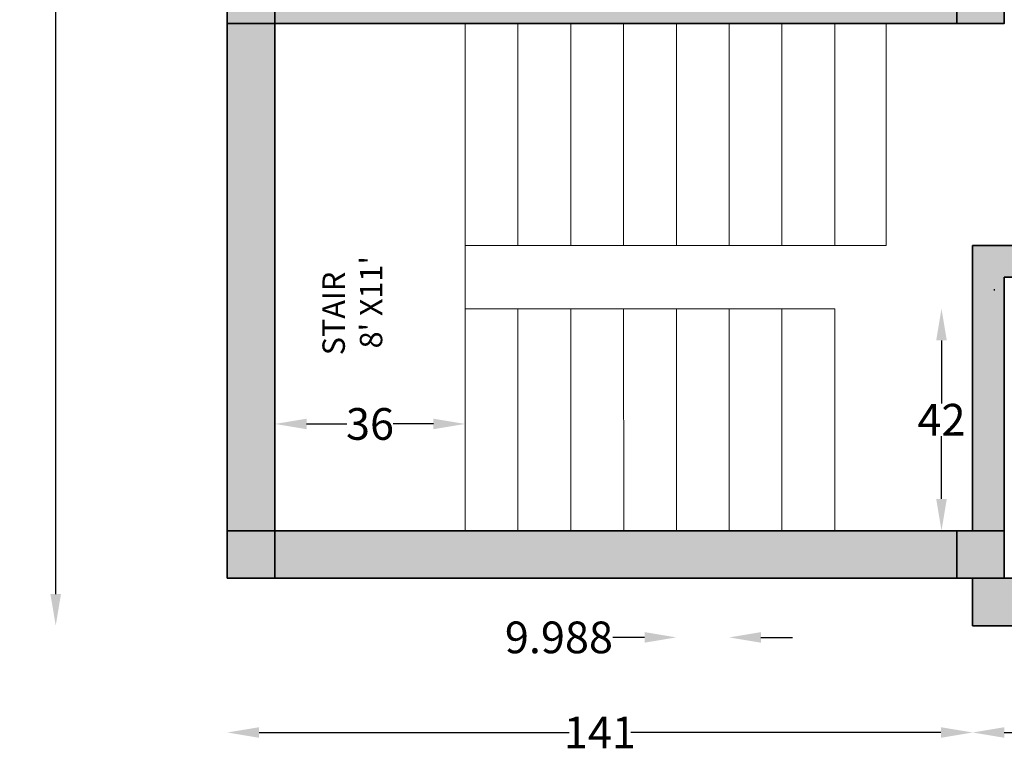
# Model space of a CAD drawing. Units: inches. Extents: x 1994 to 3075, y 3517 to 3950.
# Tile 48 of 58: x 2630 to 2816, y 3517 to 3656. Entities that reach past the tile are written whole.
import ezdxf

# ---------------------------------------------------------------- set-up
doc = ezdxf.new("R2010")
doc.units = ezdxf.units.IN
for name, color, linetype, lineweight in [('A-ANNO-DIMS', 2, 'Continuous', 18), ('A-AREA-IDEN', 7, 'Continuous', 18), ('A-COLS', 7, 'Continuous', 35), ('A-COLS-PATT', 6, 'Continuous', 13), ('A-FLOR-STRS', 7, 'Continuous', 18), ('A-WALL', 7, 'Continuous', 35), ('A-WALL-PATT', 252, 'Continuous', 13)]:
    doc.layers.add(name, color=color, linetype=linetype, lineweight=lineweight)
doc.styles.get("Standard").update_dxf_attribs({"font": 'arial.ttf'})
doc.dimstyles.get("Standard").update_dxf_attribs({"dimtxt": 6, "dimasz": 6, "dimexe": 0.18, "dimexo": 0.0625, "dimgap": 0.09, "dimtad": 0, "dimtih": 1, "dimtoh": 1, "dimdec": 4, "dimzin": 0, "dimdsep": 46, "dimlunit": 4, "dimtxsty": 'Standard', "dimcen": 0.09, "dimse1": 1, "dimse2": 1, "dimadec": 0, "dimazin": 0, "dimtfac": 1, "dimtdec": 4, "dimtofl": 0, "dimtmove": 0, "dimatfit": 3, "dimfxl": 1, "dimtolj": 1, "dimtzin": 0, "dimarcsym": 0})

# ---------------------------------------------------------------- blocks, each defined once
blk = doc.blocks.new('*D32')
at = {"layer": 'A-ANNO-DIMS', "color": 0, "lineweight": -2, "transparency": 16777216}
for p, q in [((2636.61, 3908.13), (2636.61, 3730.78)), ((2636.61, 3547.13), (2636.61, 3724.47))]:
    blk.add_line(p, q, dxfattribs=at)
at = {"layer": 'A-ANNO-DIMS', "color": 0, "transparency": 16777216}
for points in [[(2635.61, 3908.13), (2637.61, 3908.13), (2636.61, 3914.13)], [(2635.61, 3547.13), (2637.61, 3547.13), (2636.61, 3541.13)]]:
    blk.add_solid(points, dxfattribs=at)
at = {"layer": 'Defpoints', "color": 0, "transparency": 16777216}
for p in [(2636.61, 3914.13), (2669.07, 3914.13), (2810.07, 3541.13)]:
    blk.add_point(p, dxfattribs=at)
at = {"layer": 'A-ANNO-DIMS', "color": 0, "transparency": 16777216, "insert": (2636.61, 3727.63), "char_height": 6, "attachment_point": 5}
blk.add_mtext('\\A1;373', dxfattribs=at)
blk = doc.blocks.new('*D33')
at = {"layer": 'A-ANNO-DIMS', "color": 0, "lineweight": -2, "transparency": 16777216}
for p, q in [((2675.07, 3520.93), (2733.72, 3520.93)), ((2804.07, 3520.93), (2745.43, 3520.93))]:
    blk.add_line(p, q, dxfattribs=at)
at = {"layer": 'A-ANNO-DIMS', "color": 0, "transparency": 16777216}
for points in [[(2675.07, 3521.93), (2675.07, 3519.93), (2669.07, 3520.93)], [(2804.07, 3521.93), (2804.07, 3519.93), (2810.07, 3520.93)]]:
    blk.add_solid(points, dxfattribs=at)
at = {"layer": 'Defpoints', "color": 0, "transparency": 16777216}
for p in [(2669.07, 3550.13), (2810.07, 3541.13), (2810.07, 3520.93)]:
    blk.add_point(p, dxfattribs=at)
at = {"layer": 'A-ANNO-DIMS', "color": 0, "transparency": 16777216, "insert": (2739.57, 3520.93), "char_height": 6, "attachment_point": 5}
blk.add_mtext('\\A1;141', dxfattribs=at)
blk = doc.blocks.new('*D34')
at = {"layer": 'A-ANNO-DIMS', "color": 0, "lineweight": -2, "transparency": 16777216}
for p, q in [((2816.07, 3520.93), (2865.14, 3520.93)), ((2927.07, 3520.93), (2878.01, 3520.93))]:
    blk.add_line(p, q, dxfattribs=at)
at = {"layer": 'A-ANNO-DIMS', "color": 0, "transparency": 16777216}
for points in [[(2816.07, 3521.93), (2816.07, 3519.93), (2810.07, 3520.93)], [(2927.07, 3521.93), (2927.07, 3519.93), (2933.07, 3520.93)]]:
    blk.add_solid(points, dxfattribs=at)
at = {"layer": 'Defpoints', "color": 0, "transparency": 16777216}
for p in [(2810.07, 3541.13), (2933.07, 3541.13), (2933.07, 3520.93)]:
    blk.add_point(p, dxfattribs=at)
at = {"layer": 'A-ANNO-DIMS', "color": 0, "transparency": 16777216, "insert": (2871.57, 3520.93), "char_height": 6, "attachment_point": 5}
blk.add_mtext('\\A1;123', dxfattribs=at)
blk = doc.blocks.new('*D52')
at = {"layer": 'A-ANNO-DIMS', "color": 0, "lineweight": -2, "transparency": 16777216}
for p, q in [((2684.07, 3579.33), (2691.69, 3579.33)), ((2708.07, 3579.33), (2700.46, 3579.33))]:
    blk.add_line(p, q, dxfattribs=at)
at = {"layer": 'A-ANNO-DIMS', "color": 0, "transparency": 16777216}
for points in [[(2684.07, 3580.33), (2684.07, 3578.33), (2678.07, 3579.33)], [(2708.07, 3580.33), (2708.07, 3578.33), (2714.07, 3579.33)]]:
    blk.add_solid(points, dxfattribs=at)
at = {"layer": 'Defpoints', "color": 0, "transparency": 16777216}
for p in [(2714.07, 3579.33), (2678.07, 3559.13), (2714.07, 3559.13)]:
    blk.add_point(p, dxfattribs=at)
at = {"layer": 'A-ANNO-DIMS', "color": 0, "transparency": 16777216, "insert": (2696.07, 3579.33), "char_height": 6, "attachment_point": 5}
blk.add_mtext('\\A1;36', dxfattribs=at)
blk = doc.blocks.new('*D53')
at = {"layer": 'A-ANNO-DIMS', "color": 0, "lineweight": -2, "transparency": 16777216}
for p, q in [((2804.19, 3595.13), (2804.19, 3583.23)), ((2804.19, 3565.13), (2804.19, 3577.02))]:
    blk.add_line(p, q, dxfattribs=at)
at = {"layer": 'A-ANNO-DIMS', "color": 0, "transparency": 16777216}
for points in [[(2803.19, 3595.13), (2805.19, 3595.13), (2804.19, 3601.13)], [(2803.19, 3565.13), (2805.19, 3565.13), (2804.19, 3559.13)]]:
    blk.add_solid(points, dxfattribs=at)
at = {"layer": 'Defpoints', "color": 0, "transparency": 16777216}
for p in [(2783.99, 3601.13), (2783.99, 3559.13), (2804.19, 3559.13)]:
    blk.add_point(p, dxfattribs=at)
at = {"layer": 'A-ANNO-DIMS', "color": 0, "transparency": 16777216, "insert": (2804.19, 3580.13), "char_height": 6, "attachment_point": 5}
blk.add_mtext('\\A1;42', dxfattribs=at)
blk = doc.blocks.new('*D54')
at = {"layer": 'A-ANNO-DIMS', "color": 0, "lineweight": -2, "transparency": 16777216}
for p, q in [((2748.03, 3538.93), (2742.03, 3538.93)), ((2770.01, 3538.93), (2776.01, 3538.93))]:
    blk.add_line(p, q, dxfattribs=at)
at = {"layer": 'A-ANNO-DIMS', "color": 0, "transparency": 16777216}
for points in [[(2748.03, 3539.93), (2748.03, 3537.93), (2754.03, 3538.93)], [(2770.01, 3539.93), (2770.01, 3537.93), (2764.01, 3538.93)]]:
    blk.add_solid(points, dxfattribs=at)
at = {"layer": 'Defpoints', "color": 0, "transparency": 16777216}
for p in [(2754.03, 3559.13), (2764.01, 3559.13), (2754.03, 3538.93)]:
    blk.add_point(p, dxfattribs=at)
at = {"layer": 'A-ANNO-DIMS', "color": 0, "transparency": 16777216, "insert": (2731.81, 3538.93), "char_height": 6, "attachment_point": 5}
blk.add_mtext('\\A1;9.988', dxfattribs=at)
blk = doc.blocks.new('*D56')
at = {"layer": 'A-ANNO-DIMS', "color": 0, "lineweight": -2, "transparency": 16777216}
for p, q in [((2814.1, 3604.74), (2814.28, 3604.74)), ((2814.19, 3604.65), (2814.19, 3604.83)), ((2845.41, 3585.23), (2838.79, 3589.37)), ((2851.41, 3585.23), (2845.41, 3585.23))]:
    blk.add_line(p, q, dxfattribs=at)
at = {"layer": 'A-ANNO-DIMS', "color": 0, "transparency": 16777216}
blk.add_solid([(2839.32, 3590.22), (2838.26, 3588.52), (2833.7, 3592.55)], dxfattribs=at)
at = {"layer": 'Defpoints', "color": 0, "transparency": 16777216}
for p in [(2814.19, 3604.74), (2833.7, 3592.55)]:
    blk.add_point(p, dxfattribs=at)
at = {"layer": 'A-ANNO-DIMS', "color": 0, "transparency": 16777216, "insert": (2870.41, 3585.23), "char_height": 6, "attachment_point": 5}
blk.add_mtext('\\A1;2X R23.01', dxfattribs=at)

msp = doc.modelspace()

# ---------------------------------------------------------------- hatches: boundary and pattern name
at = {"layer": 'A-COLS-PATT'}
h = msp.add_hatch(color=256, dxfattribs=at)
h.dxf.hatch_style = 1
h.paths.add_polyline_path([(2678.072, 3914.1269), (2669.072, 3914.1269), (2669.072, 3905.1269), (2678.072, 3905.1269)])
h.paths.add_polyline_path([(2816.072, 3914.1269), (2807.072, 3914.1269), (2807.072, 3905.1269), (2816.072, 3905.1269)])
h.paths.add_polyline_path([(2894.9096, 3914.1269), (2885.9096, 3914.1269), (2885.9096, 3905.1269), (2894.9096, 3905.1269)])
h.paths.add_polyline_path([(3033.072, 3914.1269), (3024.072, 3914.1269), (3024.072, 3905.1269), (3033.072, 3905.1269)])
h.paths.add_polyline_path([(3033.072, 3764.1269), (3024.072, 3764.1269), (3024.072, 3755.1269), (3033.072, 3755.1269)])
h.paths.add_polyline_path([(2895.072, 3764.1269), (2886.072, 3764.1269), (2886.072, 3755.1269), (2895.072, 3755.1269)])
h.paths.add_polyline_path([(2816.072, 3764.1269), (2807.072, 3764.1269), (2807.072, 3755.1269), (2816.072, 3755.1269)])
h.paths.add_polyline_path([(2678.072, 3764.1269), (2669.072, 3764.1269), (2669.072, 3755.1269), (2678.072, 3755.1269)])
h.paths.add_polyline_path([(2678.072, 3664.1269), (2669.072, 3664.1269), (2669.072, 3655.1269), (2678.072, 3655.1269)])
h.paths.add_polyline_path([(2816.072, 3664.1269), (2807.072, 3664.1269), (2807.072, 3655.1269), (2816.072, 3655.1269)])
h.paths.add_polyline_path([(3033.072, 3616.1269), (3024.072, 3616.1269), (3024.072, 3607.1269), (3033.072, 3607.1269)])
h.paths.add_polyline_path([(2894.9096, 3616.1269), (2885.9096, 3616.1269), (2885.9096, 3607.1269), (2894.9096, 3607.1269)])
h.paths.add_polyline_path([(2816.072, 3559.1269), (2807.072, 3559.1269), (2807.072, 3550.1269), (2816.072, 3550.1269)])
h.paths.add_polyline_path([(2678.072, 3559.1269), (2669.072, 3559.1269), (2669.072, 3550.1269), (2678.072, 3550.1269)])
at = {"layer": 'A-WALL-PATT'}
h = msp.add_hatch(color=256, dxfattribs=at)
h.dxf.hatch_style = 1
h.paths.add_polyline_path([(2678.072, 3755.1269), (2669.072, 3755.1269), (2669.072, 3718.5523), (2678.072, 3718.5523)])
h.paths.add_polyline_path([(2807.072, 3761.1269), (2678.072, 3761.1269), (2678.072, 3755.1269), (2807.072, 3755.1269)])
h.paths.add_polyline_path([(2678.072, 3812.7371), (2669.072, 3812.7371), (2669.072, 3809.7371), (2669.072, 3764.1269), (2678.072, 3764.1269)])
h.paths.add_polyline_path([(2678.072, 3905.1269), (2669.072, 3905.1269), (2669.072, 3868.7491), (2678.072, 3868.7491)])
h.paths.add_polyline_path([(2723.826, 3914.1269), (2720.826, 3914.1269), (2678.072, 3914.1269), (2678.072, 3905.1269), (2723.826, 3905.1269)])
h.paths.add_polyline_path([(2807.072, 3914.1269), (2779.838, 3914.1269), (2779.838, 3905.1269), (2807.072, 3905.1269)])
h.paths.add_polyline_path([(2837.6979, 3914.1269), (2834.6979, 3914.1269), (2820.9062, 3914.1269), (2816.072, 3914.1269), (2816.072, 3905.1269), (2837.6979, 3905.1269)])
h.paths.add_polyline_path([(2885.9096, 3914.1269), (2869.71, 3914.1269), (2869.71, 3905.1269), (2876.9183, 3905.1269), (2885.9096, 3905.1269)])
h.paths.add_polyline_path([(2933.6904, 3914.1269), (2930.6904, 3914.1269), (2894.9096, 3914.1269), (2894.9096, 3905.1269), (2933.6904, 3905.1269)])
h.paths.add_polyline_path([(3024.072, 3914.1269), (2989.7025, 3914.1269), (2989.7025, 3905.1269), (3024.072, 3905.1269)])
h.paths.add_polyline_path([(3033.072, 3905.1269), (3024.072, 3905.1269), (3024.072, 3861.4192), (3033.072, 3861.4192)])
h.paths.add_polyline_path([(3033.072, 3805.4072), (3024.072, 3805.4072), (3024.072, 3764.1269), (3033.072, 3764.1269)])
h.paths.add_polyline_path([(3033.072, 3755.1269), (3024.072, 3755.1269), (3024.072, 3732.1247), (3033.072, 3732.1247), (3033.072, 3735.1247)])
h.paths.add_polyline_path([(3024.072, 3761.1269), (2895.072, 3761.1269), (2895.072, 3755.1269), (3024.072, 3755.1269)])
h.paths.add_polyline_path([(3033.072, 3676.1126), (3024.072, 3676.1126), (3024.072, 3616.1269), (3033.072, 3616.1269)])
h.paths.add_polyline_path([(3024.072, 3613.1269), (2959.4908, 3613.1269), (2959.4908, 3607.1269), (3024.072, 3607.1269)])
h.paths.add_polyline_path([(2914.1254, 3613.1269), (2894.9096, 3613.1269), (2894.9096, 3607.1269), (2914.1254, 3607.1269)])
h.paths.add_polyline_path([(2885.9096, 3613.1269), (2852.072, 3613.1269), (2852.072, 3607.1269), (2885.9096, 3607.1269)])
h.paths.add_polyline_path([(2822.072, 3613.1269), (2810.072, 3613.1269), (2810.072, 3559.1269), (2816.072, 3559.1269), (2816.072, 3607.1269), (2822.072, 3607.1269)])
h.paths.add_polyline_path([(2933.072, 3607.1269), (2924.072, 3607.1269), (2924.072, 3550.1269), (2892.072, 3550.1269), (2816.072, 3550.1269), (2810.072, 3550.1269), (2810.072, 3541.1269), (2892.072, 3541.1269), (2933.072, 3541.1269)])
h.paths.add_polyline_path([(2807.072, 3559.1269), (2678.072, 3559.1269), (2678.072, 3550.1269), (2807.072, 3550.1269)])
h.paths.add_polyline_path([(2678.072, 3655.1269), (2669.072, 3655.1269), (2669.072, 3559.1269), (2678.072, 3559.1269)])
h.paths.add_polyline_path([(2678.072, 3686.5403), (2669.072, 3686.5403), (2669.072, 3664.1269), (2678.072, 3664.1269)])
h.paths.add_polyline_path([(2807.072, 3661.1269), (2678.072, 3661.1269), (2678.072, 3655.1269), (2807.072, 3655.1269)])
h.paths.add_polyline_path([(2816.072, 3755.1269), (2810.072, 3755.1269), (2810.072, 3703.1269), (2816.072, 3703.1269)])
h.paths.add_polyline_path([(2816.072, 3905.1269), (2810.072, 3905.1269), (2810.072, 3803.1269), (2816.072, 3803.1269), (2816.072, 3815.1269)])
h.paths.add_polyline_path([(2886.072, 3821.1269), (2852.072, 3821.1269), (2852.072, 3815.1269), (2886.072, 3815.1269)])
h.paths.add_polyline_path([(2822.072, 3821.1269), (2816.072, 3821.1269), (2816.072, 3815.1269), (2822.072, 3815.1269)])
h.paths.add_polyline_path([(2892.072, 3905.1269), (2886.072, 3905.1269), (2886.072, 3803.1269), (2892.072, 3803.1269)])

# ---------------------------------------------------------------- linework, layer by layer
at = {"layer": 'A-COLS'}
for points in [[(2669.072, 3655.1269), (2678.072, 3655.1269), (2678.072, 3664.1269), (2669.072, 3664.1269)], [(2807.072, 3655.1269), (2816.072, 3655.1269), (2816.072, 3664.1269), (2807.072, 3664.1269)], [(2669.072, 3550.1269), (2678.072, 3550.1269), (2678.072, 3559.1269), (2669.072, 3559.1269)], [(2807.072, 3550.1269), (2816.072, 3550.1269), (2816.072, 3559.1269), (2807.072, 3559.1269)]]:
    msp.add_lwpolyline(points, close=True, dxfattribs=at)
at = {"layer": 'A-FLOR-STRS'}
for p, q in [((2714.072, 3655.1269), (2714.072, 3559.1269)), ((2724.0604, 3655.1269), (2724.0604, 3613.1269)), ((2734.0487, 3655.1269), (2734.0487, 3613.1269)), ((2744.0371, 3655.1269), (2744.0524, 3613.1269)), ((2754.0254, 3655.1269), (2754.0254, 3613.1269)), ((2764.0137, 3655.1269), (2764.0137, 3613.1269)), ((2774.0021, 3655.1269), (2774.0021, 3613.1269)), ((2783.9904, 3655.1269), (2783.9904, 3613.1269)), ((2793.7111, 3655.1269), (2793.7111, 3613.1269)), ((2714.072, 3613.1269), (2793.7111, 3613.1269)), ((2714.072, 3601.1269), (2783.9904, 3601.1269)), ((2724.0604, 3601.1269), (2724.0604, 3559.6097)), ((2734.0487, 3601.1269), (2734.0487, 3559.1269)), ((2744.0567, 3601.1269), (2744.072, 3559.1269)), ((2754.0254, 3601.1269), (2754.0254, 3559.1269)), ((2764.0137, 3601.1269), (2764.0137, 3559.1269)), ((2774.0021, 3601.1269), (2774.0021, 3559.1269)), ((2783.9904, 3601.1269), (2783.9904, 3559.1269)), ((2724.0604, 3559.6097), (2724.0604, 3559.1269))]:
    msp.add_line(p, q, dxfattribs=at)
at = {"layer": 'A-WALL'}
for p, q in [((2669.072, 3914.1269), (2669.072, 3550.1269)), ((2816.072, 3667.1269), (2816.072, 3655.1269)), ((2678.072, 3655.1269), (2810.072, 3655.1269)), ((2678.072, 3655.1269), (2678.072, 3559.1269)), ((2810.072, 3655.1269), (2816.072, 3655.1269)), ((2810.072, 3559.1269), (2810.072, 3613.1269)), ((2810.072, 3613.1269), (2822.072, 3613.1269)), ((2810.072, 3613.1269), (2810.072, 3559.1269)), ((2822.072, 3607.1269), (2816.072, 3607.1269)), ((2816.072, 3607.1269), (2816.072, 3550.1269)), ((2678.072, 3559.1269), (2810.072, 3559.1269)), ((2678.072, 3550.1269), (2669.072, 3550.1269)), ((2678.072, 3550.1269), (2810.072, 3550.1269)), ((2810.072, 3550.1269), (2810.072, 3541.1269)), ((2892.072, 3550.1269), (2816.072, 3550.1269)), ((2892.072, 3541.1269), (2810.072, 3541.1269))]:
    msp.add_line(p, q, dxfattribs=at)

# ---------------------------------------------------------------- texts
at = {"layer": 'A-AREA-IDEN', "insert": (2687.0719, 3592.3295), "char_height": 4.24528, "attachment_point": 1, "rotation": 90}
msp.add_mtext_dynamic_manual_height_columns("STAIR\\P 8' X11'", width=102.693633, gutter_width=21.2264, heights=[0], dxfattribs=at)

# ---------------------------------------------------------------- dimensions: what is measured, and where the dimension line sits
at = {"layer": 'A-ANNO-DIMS'}
for base, p1, p2, angle, override, picture, middle in [((2636.6096, 3914.1269), (2810.072, 3541.1269), (2669.072, 3914.1269), 90, {"dimdec": 0, "dimlfac": 1, "dimrnd": 0, "dimzin": 0, "dimdsep": 46, "dimlunit": 2}, '*D32', (2636.6096, 3727.6269)), ((2804.1904, 3559.1269), (2783.9904, 3601.1269), (2783.9904, 3559.1269), 270, {"dimdec": 0, "dimlfac": 1, "dimrnd": 0, "dimzin": 0, "dimdsep": 46, "dimlunit": 2}, '*D53', (2804.1904, 3580.1269)), ((2754.0254, 3538.9269), (2764.0137, 3559.1269), (2754.0254, 3559.1269), 180, {"dimdec": 3, "dimlfac": 1, "dimrnd": 0, "dimzin": 0, "dimdsep": 46, "dimlunit": 2}, '*D54', (2731.8058, 3538.9269))]:
    dim = msp.add_linear_dim(base=base, p1=p1, p2=p2, angle=angle, dimstyle='Standard', override=override, dxfattribs=at)
    dim.commit()
    dim.dimension.update_dxf_attribs({"geometry": picture, "text_midpoint": middle})
dim = msp.add_radius_dim(center=(2814.1856, 3604.7434), mpoint=(2833.6982, 3592.5479), text='2X <>', dimstyle='Standard', override={"dimdec": 2, "dimlfac": 1, "dimrnd": 0, "dimzin": 0, "dimdsep": 46, "dimlunit": 2}, dxfattribs=at)
dim.commit()
dim.dimension.update_dxf_attribs({"geometry": '*D56', "text_midpoint": (2870.4084, 3585.2306), "dimtype": 164})
for base, p1, p2, picture, middle in [((2714.072, 3579.3269), (2678.072, 3559.1269), (2714.072, 3559.1269), '*D52', (2696.072, 3579.3269)), ((2810.072, 3520.9269), (2669.072, 3550.1269), (2810.072, 3541.1269), '*D33', (2739.572, 3520.9269)), ((2933.072, 3520.9269), (2810.072, 3541.1269), (2933.072, 3541.1269), '*D34', (2871.572, 3520.9269))]:
    dim = msp.add_linear_dim(base=base, p1=p1, p2=p2, dimstyle='Standard', override={"dimdec": 0, "dimlfac": 1, "dimrnd": 0, "dimzin": 0, "dimdsep": 46, "dimlunit": 2}, dxfattribs=at)
    dim.commit()
    dim.dimension.update_dxf_attribs({"geometry": picture, "text_midpoint": middle})

doc.saveas('drawing.dxf')
